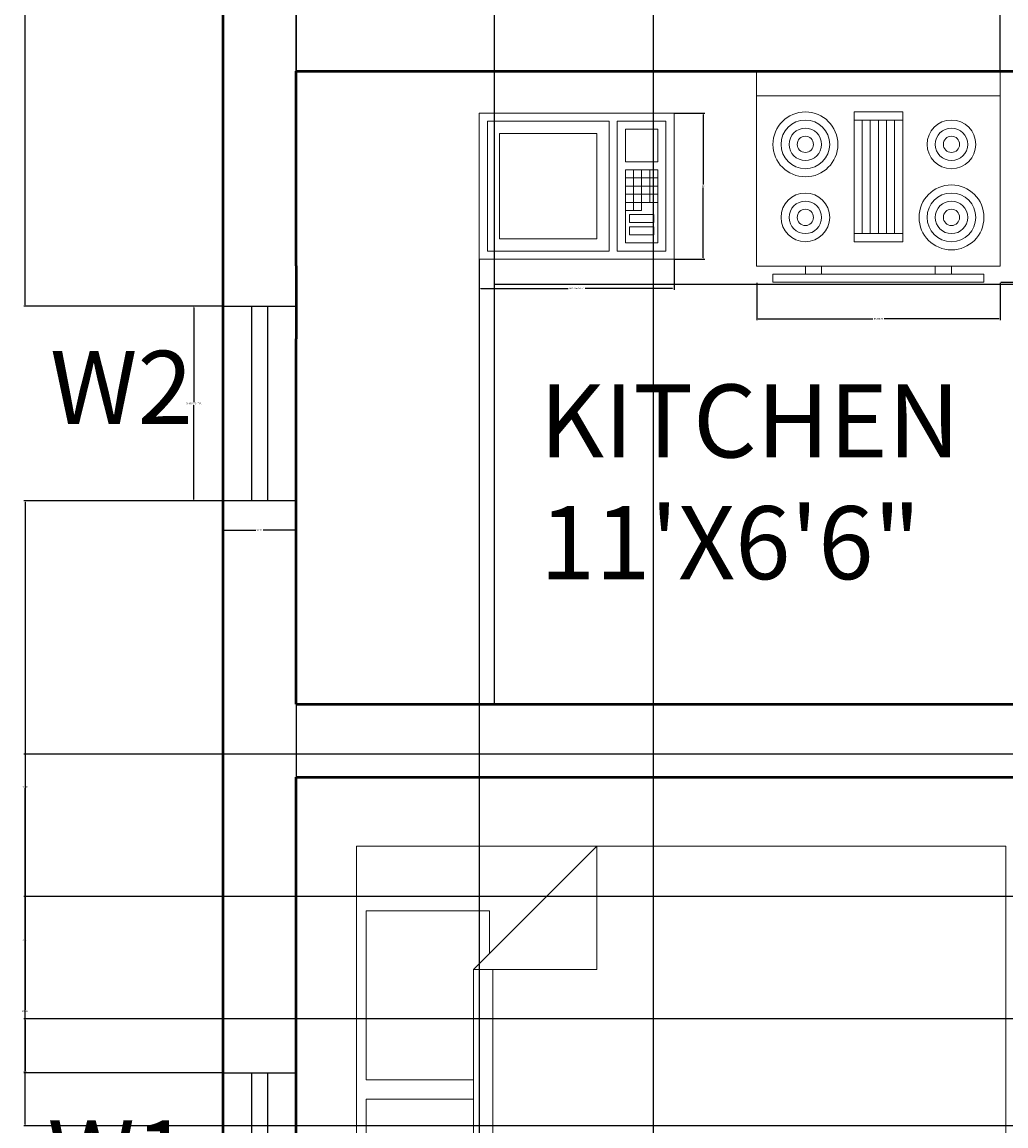
# Model space of a CAD drawing. Units: inches. Extents: x -3 to 419, y -430 to 101.
# Tile 2 of 5: x -3 to 118, y -259 to -123. Entities that reach past the tile are written whole.
import ezdxf

# ---------------------------------------------------------------- set-up
doc = ezdxf.new("R2010")
doc.units = ezdxf.units.IN
doc.header["$MEASUREMENT"] = 0
for name, color, linetype, lineweight in [('A-ANNO-DIMS', 2, 'Continuous', 18), ('A-ANNO-TEXT', 7, 'Continuous', 18), ('A-AREA-IDEN', 7, 'Continuous', 25), ('A-EQPM', 8, 'Continuous', 18), ('A-FLOR-CASE', 9, 'Continuous', 25), ('A-FURN', 8, 'Continuous', 18), ('A-GLAZ', 4, 'Continuous', 25), ('A-WALL', 7, 'Continuous', 50)]:
    doc.layers.add(name, color=color, linetype=linetype, lineweight=lineweight)
doc.styles.get("Standard").update_dxf_attribs({"font": 'arial.ttf'})
doc.dimstyles.get("Standard").update_dxf_attribs({"dimtxt": 0.18, "dimasz": 0.18, "dimexe": 0.18, "dimexo": 0.0625, "dimgap": 0.09, "dimtad": 0, "dimtih": 1, "dimtoh": 1, "dimdec": 4, "dimzin": 0, "dimdsep": 46, "dimtxsty": 'Standard', "dimcen": 0.09, "dimadec": 0, "dimazin": 0, "dimtfac": 1, "dimtdec": 4, "dimtofl": 0, "dimtmove": 0, "dimatfit": 3, "dimfxl": 1, "dimtolj": 1, "dimtzin": 0, "dimarcsym": 0})

# ---------------------------------------------------------------- blocks, each defined once
blk = doc.blocks.new('Bed - Queen')
for p, q in [((0, -80.00003), (0, 0)), ((0, 0), (59.99999, 0)), ((59.99999, 0), (59.99999, -80.00003)), ((7.99999, -1.2), (28.79998, -1.2)), ((7.99999, -14.4), (7.99999, -1.2)), ((28.79998, -1.2), (28.79998, -14.4)), ((31.19999, -1.2), (51.99999, -1.2)), ((31.19999, -14.4), (31.19999, -1.2)), ((51.99999, -1.2), (51.99999, -16.4)), ((0, -14.4), (44.8, -14.4)), ((59.99999, -29.6), (44.8, -14.4)), ((44.8, -14.4), (44.8, -29.6)), ((44.8, -16.8), (0, -16.8)), ((51.99999, -16.4), (46.79936, -16.4)), ((44.8, -29.6), (59.99999, -29.6)), ((59.99999, -80.00003), (0, -80.00003))]:
    blk.add_line(p, q)
blk = doc.blocks.new('Microwave')
for p, q in [((19, 7), (19, 11)), ((20, 11), (20, 7)), ((21, 7), (21, 11)), ((18, 10), (22, 10)), ((22, 9), (18, 9)), ((18, 8), (22, 8)), ((22, 7), (18, 7)), ((19, 6), (19, 7)), ((20, 7), (20, 6)), ((20, 6), (18, 6))]:
    blk.add_line(p, q)
for points in [[(0, 0), (0, 18), (24, 18), (24, 0)], [(1, 1), (1, 17), (16, 17), (16, 1)], [(17, 1), (17, 17), (23, 17), (23, 1)], [(2.5, 2.5), (2.5, 15.5), (14.5, 15.5), (14.5, 2.5)], [(18, 12), (18, 16), (22, 16), (22, 12)], [(18, 2), (18, 11), (22, 11), (22, 2)], [(18.5, 4.5), (18.5, 5.5), (21.5, 5.5), (21.5, 4.5)], [(18.5, 3), (18.5, 4), (21.5, 4), (21.5, 3)]]:
    blk.add_lwpolyline(points, close=True)
blk = doc.blocks.new('Range-Oven - 30 in top')
for p, q in [((0, -3), (30, -3)), ((12, -6), (18, -6)), ((13, -20), (13, -6)), ((14, -6), (14, -20)), ((15, -20), (15, -6)), ((16, -6), (16, -20)), ((17, -20), (17, -6)), ((18, -20), (12, -20)), ((6, -24), (6, -25)), ((8, -25), (8, -24)), ((22, -25), (22, -24)), ((24, -24), (24, -25))]:
    blk.add_line(p, q)
for points in [[(0, -24), (0, 0), (30, 0), (30, -24)], [(12, -21), (12, -5), (18, -5), (18, -21)], [(2, -26), (2, -25), (28, -25), (28, -26)]]:
    blk.add_lwpolyline(points, close=True)
for centre, radius in [((6, -9), 4), ((6, -9), 3), ((24, -9), 3), ((6, -9), 2), ((6, -9), 1), ((24, -9), 2), ((24, -9), 1), ((24, -18), 4), ((6, -18), 3), ((6, -18), 2), ((24, -18), 3), ((24, -18), 2), ((6, -18), 1), ((24, -18), 1)]:
    blk.add_circle(centre, radius)
blk = doc.blocks.new('WINDOW-24IN')
for p, q in [((0, 5.5), (24, 5.5)), ((0, 3.5), (24, 3.5))]:
    blk.add_line(p, q)
blk.add_lwpolyline([(0, 9), (24, 9), (24, 0), (0, 0)], close=True)
blk = doc.blocks.new('*D9')
at = {"layer": 'A-ANNO-DIMS', "color": 0, "lineweight": -2, "transparency": 16777216}
for p, q in [((21.49, -157.64), (17.77, -157.64)), ((17.95, -157.82), (17.95, -169.46)), ((17.95, -181.46), (17.95, -169.83)), ((21.49, -181.64), (17.77, -181.64))]:
    blk.add_line(p, q, dxfattribs=at)
at = {"layer": 'A-ANNO-DIMS', "color": 0, "transparency": 16777216}
for points in [[(17.92, -157.82), (17.98, -157.82), (17.95, -157.64)], [(17.92, -181.46), (17.98, -181.46), (17.95, -181.64)]]:
    blk.add_solid(points, dxfattribs=at)
at = {"layer": 'Defpoints', "color": 0, "transparency": 16777216}
for p in [(21.55, -157.64), (17.95, -181.64), (21.55, -181.64)]:
    blk.add_point(p, dxfattribs=at)
at = {"layer": 'A-ANNO-DIMS', "color": 0, "transparency": 16777216, "insert": (17.95, -169.64), "char_height": 0.18, "attachment_point": 5}
blk.add_mtext('\\A1;WINDOW 24 TYP.', dxfattribs=at)
blk = doc.blocks.new('*D10')
at = {"layer": 'A-ANNO-DIMS', "color": 0, "lineweight": -2, "transparency": 16777216}
for p, q in [((21.55, -181.71), (21.55, -185.42)), ((30.55, -181.71), (30.55, -185.42)), ((21.73, -185.24), (25.6, -185.24)), ((30.37, -185.24), (26.51, -185.24))]:
    blk.add_line(p, q, dxfattribs=at)
at = {"layer": 'A-ANNO-DIMS', "color": 0, "transparency": 16777216}
for points in [[(21.73, -185.21), (21.73, -185.27), (21.55, -185.24)], [(30.37, -185.21), (30.37, -185.27), (30.55, -185.24)]]:
    blk.add_solid(points, dxfattribs=at)
at = {"layer": 'Defpoints', "color": 0, "transparency": 16777216}
for p in [(21.55, -181.64), (30.55, -181.64), (30.55, -185.24)]:
    blk.add_point(p, dxfattribs=at)
at = {"layer": 'A-ANNO-DIMS', "color": 0, "transparency": 16777216, "insert": (26.05, -185.24), "char_height": 0.18, "attachment_point": 5}
blk.add_mtext('\\A1;9 TYP.', dxfattribs=at)
blk = doc.blocks.new('*D15')
at = {"layer": 'A-ANNO-DIMS', "color": 0, "lineweight": -2, "transparency": 16777216}
for p, q in [((53.12, -151.91), (53.12, -155.63)), ((77.12, -151.91), (77.12, -155.63)), ((53.3, -155.45), (64.09, -155.45)), ((76.94, -155.45), (66.16, -155.45))]:
    blk.add_line(p, q, dxfattribs=at)
at = {"layer": 'A-ANNO-DIMS', "color": 0, "transparency": 16777216}
for points in [[(53.3, -155.42), (53.3, -155.48), (53.12, -155.45)], [(76.94, -155.42), (76.94, -155.48), (77.12, -155.45)]]:
    blk.add_solid(points, dxfattribs=at)
at = {"layer": 'Defpoints', "color": 0, "transparency": 16777216}
for p in [(53.12, -151.85), (77.12, -151.85), (77.12, -155.45)]:
    blk.add_point(p, dxfattribs=at)
at = {"layer": 'A-ANNO-DIMS', "color": 0, "transparency": 16777216, "insert": (65.12, -155.45), "char_height": 0.18, "attachment_point": 5}
blk.add_mtext('\\A1;MICROWAVE 24', dxfattribs=at)
blk = doc.blocks.new('*D16')
at = {"layer": 'A-ANNO-DIMS', "color": 0, "lineweight": -2, "transparency": 16777216}
for p, q in [((77.19, -133.85), (80.9, -133.85)), ((80.72, -134.03), (80.72, -142.66)), ((80.72, -151.67), (80.72, -143.03)), ((77.19, -151.85), (80.9, -151.85))]:
    blk.add_line(p, q, dxfattribs=at)
at = {"layer": 'A-ANNO-DIMS', "color": 0, "transparency": 16777216}
for points in [[(80.69, -134.03), (80.75, -134.03), (80.72, -133.85)], [(80.69, -151.67), (80.75, -151.67), (80.72, -151.85)]]:
    blk.add_solid(points, dxfattribs=at)
at = {"layer": 'Defpoints', "color": 0, "transparency": 16777216}
for p in [(77.12, -133.85), (80.72, -133.85), (77.12, -151.85)]:
    blk.add_point(p, dxfattribs=at)
at = {"layer": 'A-ANNO-DIMS', "color": 0, "transparency": 16777216, "insert": (80.72, -142.85), "char_height": 0.18, "attachment_point": 5}
blk.add_mtext('\\A1;18', dxfattribs=at)
blk = doc.blocks.new('*D17')
at = {"layer": 'A-ANNO-DIMS', "color": 0, "lineweight": -2, "transparency": 16777216}
for p, q in [((87.3, -154.76), (87.3, -159.38)), ((117.3, -154.76), (117.3, -159.38)), ((87.48, -159.2), (101.6, -159.2)), ((117.12, -159.2), (103, -159.2))]:
    blk.add_line(p, q, dxfattribs=at)
at = {"layer": 'A-ANNO-DIMS', "color": 0, "transparency": 16777216}
for points in [[(87.48, -159.17), (87.48, -159.23), (87.3, -159.2)], [(117.12, -159.17), (117.12, -159.23), (117.3, -159.2)]]:
    blk.add_solid(points, dxfattribs=at)
at = {"layer": 'Defpoints', "color": 0, "transparency": 16777216}
for p in [(87.3, -154.7), (117.3, -154.7), (117.3, -159.2)]:
    blk.add_point(p, dxfattribs=at)
at = {"layer": 'A-ANNO-DIMS', "color": 0, "transparency": 16777216, "insert": (102.3, -159.2), "char_height": 0.18, "attachment_point": 5}
blk.add_mtext('\\A1;RANGE 30', dxfattribs=at)
blk = doc.blocks.new('*D18')
at = {"layer": 'A-ANNO-DIMS', "color": 0, "lineweight": -2, "transparency": 16777216}
for p, q in [((117.36, -128.7), (121.98, -128.7)), ((121.8, -128.88), (121.8, -141.52)), ((121.8, -154.52), (121.8, -141.88)), ((117.36, -154.7), (121.98, -154.7))]:
    blk.add_line(p, q, dxfattribs=at)
at = {"layer": 'A-ANNO-DIMS', "color": 0, "transparency": 16777216}
for points in [[(121.77, -128.88), (121.83, -128.88), (121.8, -128.7)], [(121.77, -154.52), (121.83, -154.52), (121.8, -154.7)]]:
    blk.add_solid(points, dxfattribs=at)
at = {"layer": 'Defpoints', "color": 0, "transparency": 16777216}
for p in [(117.3, -128.7), (121.8, -128.7), (117.3, -154.7)]:
    blk.add_point(p, dxfattribs=at)
at = {"layer": 'A-ANNO-DIMS', "color": 0, "transparency": 16777216, "insert": (121.8, -141.7), "char_height": 0.18, "attachment_point": 5}
blk.add_mtext('\\A1;26', dxfattribs=at)
blk = doc.blocks.new('*D28')
at = {"layer": 'A-ANNO-DIMS', "color": 0, "lineweight": -2, "transparency": 16777216}
for p, q in [((21.49, 21.31), (-3, 21.31)), ((-2.82, 21.13), (-2.82, -67.98)), ((-2.82, -157.46), (-2.82, -68.35)), ((21.49, -157.64), (-3, -157.64))]:
    blk.add_line(p, q, dxfattribs=at)
at = {"layer": 'A-ANNO-DIMS', "color": 0, "transparency": 16777216}
for points in [[(-2.85, 21.13), (-2.79, 21.13), (-2.82, 21.31)], [(-2.85, -157.46), (-2.79, -157.46), (-2.82, -157.64)]]:
    blk.add_solid(points, dxfattribs=at)
at = {"layer": 'Defpoints', "color": 0, "transparency": 16777216}
for p in [(21.55, 21.31), (-2.82, -157.64), (21.55, -157.64)]:
    blk.add_point(p, dxfattribs=at)
at = {"layer": 'A-ANNO-DIMS', "color": 0, "transparency": 16777216, "insert": (-2.82, -68.16), "char_height": 0.18, "attachment_point": 5}
blk.add_mtext('\\A1;178.96', dxfattribs=at)
blk = doc.blocks.new('*D29')
at = {"layer": 'A-ANNO-DIMS', "color": 0, "lineweight": -2, "transparency": 16777216}
for p, q in [((21.49, -181.64), (-3, -181.64)), ((-2.82, -181.82), (-2.82, -216.71)), ((-2.82, -251.95), (-2.82, -217.07)), ((21.49, -252.13), (-3, -252.13))]:
    blk.add_line(p, q, dxfattribs=at)
at = {"layer": 'A-ANNO-DIMS', "color": 0, "transparency": 16777216}
for points in [[(-2.85, -181.82), (-2.79, -181.82), (-2.82, -181.64)], [(-2.85, -251.95), (-2.79, -251.95), (-2.82, -252.13)]]:
    blk.add_solid(points, dxfattribs=at)
at = {"layer": 'Defpoints', "color": 0, "transparency": 16777216}
for p in [(21.55, -181.64), (-2.82, -252.13), (21.55, -252.13)]:
    blk.add_point(p, dxfattribs=at)
at = {"layer": 'A-ANNO-DIMS', "color": 0, "transparency": 16777216, "insert": (-2.82, -216.89), "char_height": 0.18, "attachment_point": 5}
blk.add_mtext('\\A1;70.49', dxfattribs=at)
blk = doc.blocks.new('*D40')
at = {"layer": 'A-ANNO-DIMS', "color": 0, "lineweight": -2, "transparency": 16777216}
for p, q in [((171.49, -245.49), (-3, -245.49)), ((-2.82, -245.67), (-2.82, -251.9)), ((-2.82, -258.51), (-2.82, -252.27)), ((171.49, -258.69), (-3, -258.69))]:
    blk.add_line(p, q, dxfattribs=at)
at = {"layer": 'A-ANNO-DIMS', "color": 0, "transparency": 16777216}
for points in [[(-2.85, -245.67), (-2.79, -245.67), (-2.82, -245.49)], [(-2.85, -258.51), (-2.79, -258.51), (-2.82, -258.69)]]:
    blk.add_solid(points, dxfattribs=at)
at = {"layer": 'Defpoints', "color": 0, "transparency": 16777216}
for p in [(171.55, -245.49), (-2.82, -258.69), (171.55, -258.69)]:
    blk.add_point(p, dxfattribs=at)
at = {"layer": 'A-ANNO-DIMS', "color": 0, "transparency": 16777216, "insert": (-2.82, -252.09), "char_height": 0.18, "attachment_point": 5}
blk.add_mtext('\\A1;13.2', dxfattribs=at)
blk = doc.blocks.new('*D48')
at = {"layer": 'A-ANNO-DIMS', "color": 0, "lineweight": -2, "transparency": 16777216}
for p, q in [((30.55, -128.62), (30.55, 101.37)), ((30.73, 101.19), (83.19, 101.19)), ((136.55, 101.19), (84.1, 101.19)), ((136.73, -128.62), (136.73, 101.37))]:
    blk.add_line(p, q, dxfattribs=at)
at = {"layer": 'A-ANNO-DIMS', "color": 0, "transparency": 16777216}
for points in [[(30.73, 101.22), (30.73, 101.16), (30.55, 101.19)], [(136.55, 101.22), (136.55, 101.16), (136.73, 101.19)]]:
    blk.add_solid(points, dxfattribs=at)
at = {"layer": 'Defpoints', "color": 0, "transparency": 16777216}
for p in [(136.73, 101.19), (30.55, -128.69), (136.73, -128.69)]:
    blk.add_point(p, dxfattribs=at)
at = {"layer": 'A-ANNO-DIMS', "color": 0, "transparency": 16777216, "insert": (83.64, 101.19), "char_height": 0.18, "attachment_point": 5}
blk.add_mtext('\\A1;106.18', dxfattribs=at)
blk = doc.blocks.new('*D49')
at = {"layer": 'A-ANNO-DIMS', "color": 0, "lineweight": -2, "transparency": 16777216}
for p, q in [((30.55, -206.62), (30.55, 101.37)), ((30.73, 101.19), (42.38, 101.19)), ((54.82, 101.19), (43.17, 101.19)), ((55, -206.62), (55, 101.37))]:
    blk.add_line(p, q, dxfattribs=at)
at = {"layer": 'A-ANNO-DIMS', "color": 0, "transparency": 16777216}
for points in [[(30.73, 101.22), (30.73, 101.16), (30.55, 101.19)], [(54.82, 101.22), (54.82, 101.16), (55, 101.19)]]:
    blk.add_solid(points, dxfattribs=at)
at = {"layer": 'Defpoints', "color": 0, "transparency": 16777216}
for p in [(55, 101.19), (30.55, -206.69), (55, -206.69)]:
    blk.add_point(p, dxfattribs=at)
at = {"layer": 'A-ANNO-DIMS', "color": 0, "transparency": 16777216, "insert": (42.78, 101.19), "char_height": 0.18, "attachment_point": 5}
blk.add_mtext('\\A1;24.45', dxfattribs=at)
blk = doc.blocks.new('*D51')
at = {"layer": 'A-ANNO-DIMS', "color": 0, "lineweight": -2, "transparency": 16777216}
for p, q in [((53.12, -151.91), (53.12, -429.67)), ((30.55, -157.71), (30.55, -429.67)), ((30.73, -429.49), (41.44, -429.49)), ((52.94, -429.49), (42.23, -429.49))]:
    blk.add_line(p, q, dxfattribs=at)
at = {"layer": 'A-ANNO-DIMS', "color": 0, "transparency": 16777216}
for points in [[(30.73, -429.46), (30.73, -429.52), (30.55, -429.49)], [(52.94, -429.46), (52.94, -429.52), (53.12, -429.49)]]:
    blk.add_solid(points, dxfattribs=at)
at = {"layer": 'Defpoints', "color": 0, "transparency": 16777216}
for p in [(53.12, -151.85), (30.55, -157.64), (30.55, -429.49)]:
    blk.add_point(p, dxfattribs=at)
at = {"layer": 'A-ANNO-DIMS', "color": 0, "transparency": 16777216, "insert": (41.84, -429.49), "char_height": 0.18, "attachment_point": 5}
blk.add_mtext('\\A1;22.57', dxfattribs=at)
blk = doc.blocks.new('*D52')
at = {"layer": 'A-ANNO-DIMS', "color": 0, "lineweight": -2, "transparency": 16777216}
for p, q in [((117.3, -128.64), (117.3, 101.37)), ((117.48, 101.19), (126.63, 101.19)), ((136.55, 101.19), (127.4, 101.19)), ((136.73, -128.62), (136.73, 101.37))]:
    blk.add_line(p, q, dxfattribs=at)
at = {"layer": 'A-ANNO-DIMS', "color": 0, "transparency": 16777216}
for points in [[(117.48, 101.22), (117.48, 101.16), (117.3, 101.19)], [(136.55, 101.22), (136.55, 101.16), (136.73, 101.19)]]:
    blk.add_solid(points, dxfattribs=at)
at = {"layer": 'Defpoints', "color": 0, "transparency": 16777216}
for p in [(136.73, 101.19), (117.3, -128.7), (136.73, -128.69)]:
    blk.add_point(p, dxfattribs=at)
at = {"layer": 'A-ANNO-DIMS', "color": 0, "transparency": 16777216, "insert": (127.01, 101.19), "char_height": 0.18, "attachment_point": 5}
blk.add_mtext('\\A1;19.43', dxfattribs=at)
blk = doc.blocks.new('*D54')
at = {"layer": 'A-ANNO-DIMS', "color": 0, "lineweight": -2, "transparency": 16777216}
for p, q in [((201.4, -230.4), (-3, -230.4)), ((-2.82, -230.58), (-2.82, -244.36)), ((-2.82, -258.51), (-2.82, -244.72)), ((199.03, -258.69), (-3, -258.69))]:
    blk.add_line(p, q, dxfattribs=at)
at = {"layer": 'A-ANNO-DIMS', "color": 0, "transparency": 16777216}
for points in [[(-2.85, -230.58), (-2.79, -230.58), (-2.82, -230.4)], [(-2.85, -258.51), (-2.79, -258.51), (-2.82, -258.69)]]:
    blk.add_solid(points, dxfattribs=at)
at = {"layer": 'Defpoints', "color": 0, "transparency": 16777216}
for p in [(201.46, -230.4), (-2.82, -258.69), (199.09, -258.69)]:
    blk.add_point(p, dxfattribs=at)
at = {"layer": 'A-ANNO-DIMS', "color": 0, "transparency": 16777216, "insert": (-2.82, -244.54), "char_height": 0.18, "attachment_point": 5}
blk.add_mtext('\\A1;28.286', dxfattribs=at)
blk = doc.blocks.new('*D55')
at = {"layer": 'A-ANNO-DIMS', "color": 0, "lineweight": -2, "transparency": 16777216}
for p, q in [((255.33, -212.85), (-3, -212.85)), ((-2.82, -213.03), (-2.82, -235.59)), ((-2.82, -258.51), (-2.82, -235.95)), ((269.16, -258.69), (-3, -258.69))]:
    blk.add_line(p, q, dxfattribs=at)
at = {"layer": 'A-ANNO-DIMS', "color": 0, "transparency": 16777216}
for points in [[(-2.85, -213.03), (-2.79, -213.03), (-2.82, -212.85)], [(-2.85, -258.51), (-2.79, -258.51), (-2.82, -258.69)]]:
    blk.add_solid(points, dxfattribs=at)
at = {"layer": 'Defpoints', "color": 0, "transparency": 16777216}
for p in [(255.4, -212.85), (-2.82, -258.69), (269.22, -258.69)]:
    blk.add_point(p, dxfattribs=at)
at = {"layer": 'A-ANNO-DIMS', "color": 0, "transparency": 16777216, "insert": (-2.82, -235.77), "char_height": 0.18, "attachment_point": 5}
blk.add_mtext('\\A1;45.83', dxfattribs=at)
blk = doc.blocks.new('*D59')
at = {"layer": 'A-ANNO-DIMS', "color": 0, "lineweight": -2, "transparency": 16777216}
for p, q in [((30.55, 12.25), (30.55, -429.67)), ((74.54, 7.17), (74.54, -429.67)), ((30.73, -429.49), (52.15, -429.49)), ((74.36, -429.49), (52.95, -429.49))]:
    blk.add_line(p, q, dxfattribs=at)
at = {"layer": 'A-ANNO-DIMS', "color": 0, "transparency": 16777216}
for points in [[(30.73, -429.46), (30.73, -429.52), (30.55, -429.49)], [(74.36, -429.46), (74.36, -429.52), (74.54, -429.49)]]:
    blk.add_solid(points, dxfattribs=at)
at = {"layer": 'Defpoints', "color": 0, "transparency": 16777216}
for p in [(30.55, 12.31), (74.54, 7.23), (74.54, -429.49)]:
    blk.add_point(p, dxfattribs=at)
at = {"layer": 'A-ANNO-DIMS', "color": 0, "transparency": 16777216, "insert": (52.55, -429.49), "char_height": 0.18, "attachment_point": 5}
blk.add_mtext('\\A1;43.99', dxfattribs=at)

msp = doc.modelspace()

# ---------------------------------------------------------------- linework, layer by layer
at = {"layer": 'A-FLOR-CASE'}
for p, q in [((55.004, -206.6853), (55.004, -154.9237)), ((55.004, -154.9237), (136.73, -154.9237))]:
    msp.add_line(p, q, dxfattribs=at)
at = {"layer": 'A-WALL'}
for p, q in [((30.5532, -152.6853), (30.5532, -128.6853)), ((30.5532, -128.6853), (162.5532, -128.6853)), ((30.5532, -152.6853), (30.5532, -161.6853)), ((30.5532, -206.6853), (30.5532, -161.6853)), ((30.5532, -206.6853), (162.5532, -206.6853)), ((30.5532, -286.6853), (30.5532, -215.6853)), ((30.5532, -215.6853), (162.5532, -215.6853))]:
    msp.add_line(p, q, dxfattribs=at)
msp.add_lwpolyline([(266.5221, -404.6853), (21.5532, -404.6853), (21.5532, 21.3147), (345.5532, 21.3147), (345.5532, -404.6853)], dxfattribs=at)

# ---------------------------------------------------------------- block references
at = {"layer": 'A-EQPM'}
for name, p in [('Range-Oven - 30 in top', (87.2993, -128.7009)), ('Microwave', (53.124, -151.8457))]:
    msp.add_blockref(name, p, dxfattribs=at)
at = {"layer": 'A-FURN', "rotation": 90}
msp.add_blockref('Bed - Queen', (38.0056, -284.1853), dxfattribs=at)
at = {"layer": 'A-GLAZ'}
for p, rotation in [((21.5535, -157.6433), 270), ((21.5535, -252.131), 269.9999999999999)]:
    msp.add_blockref('WINDOW-24IN', p, dxfattribs=dict(at, rotation=rotation))

# ---------------------------------------------------------------- texts
at = {"layer": 'A-ANNO-TEXT', "char_height": 9, "attachment_point": 1}
for s, width, insert in [('W2', 31.337154, (0.2411, -163.1493)), ('W1', 37.451717, (-0.0716, -258.0081))]:
    msp.add_mtext_dynamic_manual_height_columns(s, width=width, gutter_width=45, heights=[0], dxfattribs=dict(at, insert=insert))
at = {"layer": 'A-AREA-IDEN', "insert": (60.5763, -167.2919), "char_height": 9, "attachment_point": 1}
msp.add_mtext_dynamic_manual_height_columns('KITCHEN\\P11\'X6\'6"', width=56.650984, gutter_width=45, heights=[0], dxfattribs=at)

# ---------------------------------------------------------------- dimensions: what is measured, and where the dimension line sits
at = {"layer": 'A-ANNO-DIMS'}
for base, p1, p2, picture, middle in [((136.73, 101.1903), (30.5532, -128.6853), (136.73, -128.6853), '*D48', (83.6416, 101.1903)), ((55.004, 101.1903), (30.5532, -206.6853), (55.004, -206.6853), '*D49', (42.7786, 101.1903)), ((136.73, 101.1903), (117.2993, -128.7009), (136.73, -128.6853), '*D52', (127.0147, 101.1903)), ((74.5439, -429.4854), (30.5532, 12.3147), (74.5439, 7.23), '*D59', (52.5485, -429.4854)), ((30.5532, -429.4854), (53.124, -151.8457), (30.5532, -157.6432), '*D51', (41.8386, -429.4854))]:
    dim = msp.add_linear_dim(base=base, p1=p1, p2=p2, dimstyle='Standard', override={"dimdec": 2, "dimlfac": 1, "dimrnd": 0, "dimzin": 0, "dimdsep": 46, "dimlunit": 2}, dxfattribs=at)
    dim.commit()
    dim.dimension.update_dxf_attribs({"geometry": picture, "text_midpoint": middle})
for base, p1, p2, override, picture, middle in [((-2.8238, -157.6432), (21.5532, 21.3147), (21.5532, -157.6432), {"dimdec": 2, "dimlfac": 1, "dimrnd": 0, "dimzin": 0, "dimdsep": 46, "dimlunit": 2}, '*D28', (-2.8238, -68.1642)), ((121.7993, -128.7009), (117.2993, -154.7009), (117.2993, -128.7009), {"dimdec": 0, "dimlfac": 1, "dimrnd": 0, "dimzin": 0, "dimdsep": 46, "dimlunit": 2}, '*D18', (121.7993, -141.7009)), ((80.724, -133.8457), (77.124, -151.8457), (77.124, -133.8457), {"dimdec": 0, "dimlfac": 1, "dimrnd": 0, "dimzin": 0, "dimdsep": 46, "dimlunit": 2}, '*D16', (80.724, -142.8457)), ((-2.8238, -252.1309), (21.5532, -181.6432), (21.5532, -252.1309), {"dimdec": 2, "dimlfac": 1, "dimrnd": 0, "dimzin": 0, "dimdsep": 46, "dimlunit": 2}, '*D29', (-2.8238, -216.887)), ((-2.8238, -258.6853), (255.3974, -212.8529), (269.2198, -258.6853), {"dimdec": 2, "dimlfac": 1, "dimrnd": 0, "dimzin": 0, "dimdsep": 46, "dimlunit": 2}, '*D55', (-2.8238, -235.7691)), ((-2.82381, -258.68531), (201.45976, -230.39884), (199.09163, -258.68531), {"dimdec": 3, "dimlfac": 1, "dimrnd": 0, "dimzin": 0, "dimdsep": 46, "dimlunit": 2}, '*D54', (-2.82381, -244.54208)), ((-2.8238, -258.6853), (171.5532, -245.4865), (171.5532, -258.6853), {"dimdec": 1, "dimlfac": 1, "dimrnd": 0, "dimzin": 0, "dimdsep": 46, "dimlunit": 2}, '*D40', (-2.8238, -252.0859))]:
    dim = msp.add_linear_dim(base=base, p1=p1, p2=p2, angle=90, dimstyle='Standard', override=override, dxfattribs=at)
    dim.commit()
    dim.dimension.update_dxf_attribs({"geometry": picture, "text_midpoint": middle})
for base, p1, p2, text, picture, middle in [((77.124, -155.4457), (53.124, -151.8457), (77.124, -151.8457), 'MICROWAVE <>', '*D15', (65.124, -155.4457)), ((117.2993, -159.2009), (87.2993, -154.7009), (117.2993, -154.7009), 'RANGE <>', '*D17', (102.2993, -159.2009)), ((30.5532, -185.2432), (21.5532, -181.6432), (30.5532, -181.6432), '<> TYP.', '*D10', (26.0532, -185.2432))]:
    dim = msp.add_linear_dim(base=base, p1=p1, p2=p2, text=text, dimstyle='Standard', override={"dimdec": 0, "dimlfac": 1, "dimrnd": 0, "dimzin": 0, "dimdsep": 46, "dimlunit": 2}, dxfattribs=at)
    dim.commit()
    dim.dimension.update_dxf_attribs({"geometry": picture, "text_midpoint": middle})
dim = msp.add_linear_dim(base=(17.9532, -181.6432), p1=(21.5532, -157.6432), p2=(21.5532, -181.6432), angle=270, text='WINDOW <> TYP.', dimstyle='Standard', override={"dimdec": 0, "dimlfac": 1, "dimrnd": 0, "dimzin": 0, "dimdsep": 46, "dimlunit": 2}, dxfattribs=at)
dim.commit()
dim.dimension.update_dxf_attribs({"geometry": '*D9', "text_midpoint": (17.9532, -169.6432)})

doc.saveas('drawing.dxf')
